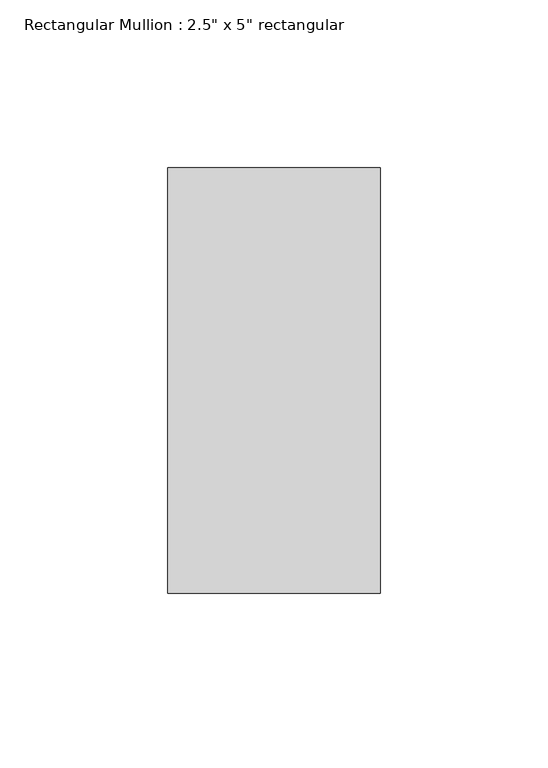
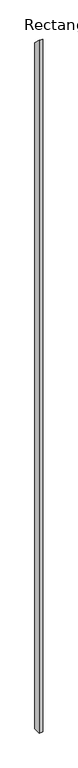
"""IFC4 building model written with IfcOpenShell, lengths in millimetres: member geometry."""

from ifc_helpers import new_model, si_unit, frame, origin, place, context, project, spatial, polyline, outline, extrude, source, transform, mapped, element, save


def member_b46abd34(model_context):
    return source(origin(), model_context, "Body", "SweptSolid", [
        extrude(outline(polyline([(-63.5, 63.5), (63.5, -63.5), (63.5, -12735.3989237), (-63.5, -12735.3989237), (-63.5, 63.5)])), frame((-63.5, 0.0, 0.0), z_axis=(1.0, 0.0, 0.0), x_axis=(0.0, 1.0, 0.0)), (0.0, 0.0, 1.0), 63.5),
    ])


if __name__ == "__main__":
    model = new_model("IFC4")
    model_context = context("Model", 3, world=origin())
    ifc_project = project(units=[si_unit("LENGTHUNIT", "METRE", prefix="MILLI")], contexts=[model_context])
    site = spatial("IfcSite", under=ifc_project)
    building = spatial("IfcBuilding", under=site)
    placement = place(None, origin())
    member_shape = member_b46abd34(model_context)
    element("IfcMember", 1, ObjectType="Rectangular Mullion : 2.5\" x 5\" rectangular", at=placement, inside=building, context=model_context, shape_type="MappedRepresentation", body=[
        mapped(member_shape, transform((0.0, 0.0, 0.0), x_axis=(1.0, 0.0, 0.0), y_axis=(0.0, 1.0, 0.0), z_axis=(0.0, 0.0, 1.0))),
    ])
    save(model, "model.ifc")

# Revit data of these elements
# Type "Rectangular Mullion : 2.5\" x 5\" rectangular"
#   built-in parameter 1007304 = 0.416667 (stored number, unit not read)
#   built-in parameter 1007301 = 0.104167 (stored number, unit not read)
#   built-in parameter 1007300 = 0.104167 (stored number, unit not read)
# Element 1 (IfcMember, "Rectangular Mullion : 2.5\" x 5\" rectangular")
#   Materials on its faces: "Aluminum"
# Materials
#   "Aluminum": class "Metal", colour RGB 247 247 247, transparency 0, Description = "Aluminum 6061", Cost = 0
